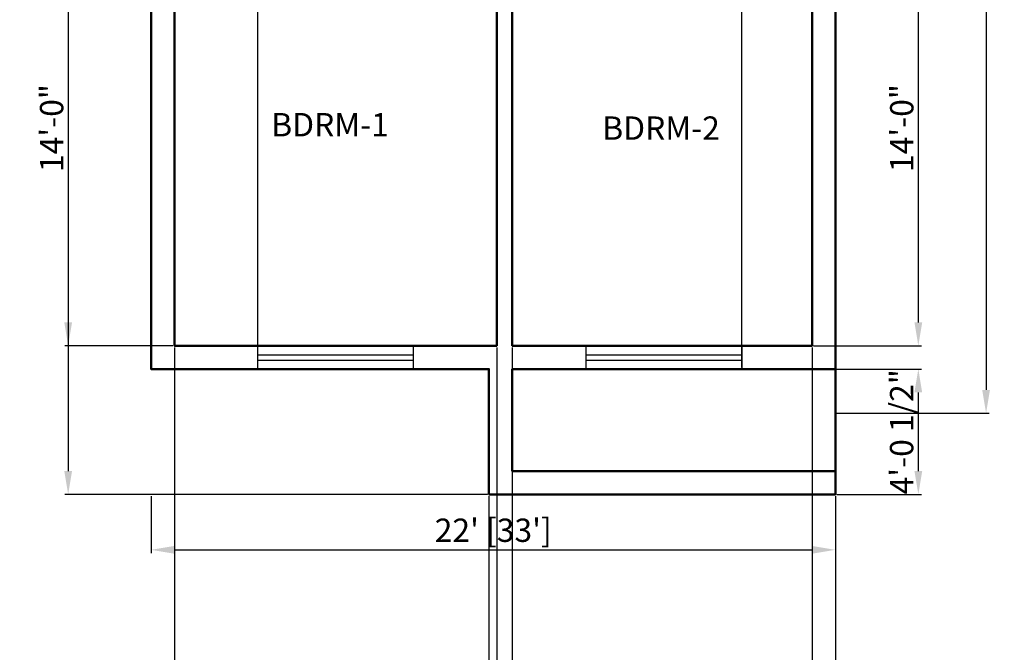
# Model space of a CAD drawing. Units: inches. Extents: x 2429 to 3343, y 1496 to 2530.
# Tile 5 of 7: x 2954 to 3334, y 1910 to 2154. Entities that reach past the tile are written whole.
import ezdxf

# ---------------------------------------------------------------- set-up
doc = ezdxf.new("R2010")
doc.units = ezdxf.units.IN
for name, color, linetype, lineweight in [('A-ANNO-DIMS', 2, 'Continuous', 18), ('A-AREA-IDEN', 3, 'Continuous', 18), ('A-GLAZ', 4, 'Continuous', 25), ('A-WALL', 7, 'Continuous', 50)]:
    doc.layers.add(name, color=color, linetype=linetype, lineweight=lineweight)
doc.styles.get("Standard").update_dxf_attribs({"font": 'arial.ttf'})
doc.dimstyles.new('ISO-25', dxfattribs={"dimtxt": 9, "dimasz": 9, "dimexe": 1.25, "dimexo": 0.625, "dimtad": 1, "dimdec": 1, "dimlunit": 3, "dimtxsty": 'Standard', "dimcen": 9, "dimadec": 0, "dimazin": 0, "dimtfac": 1, "dimtdec": 1, "dimtmove": 0, "dimatfit": 3, "dimfxl": 1, "dimarcsym": 0})

# ---------------------------------------------------------------- blocks, each defined once
blk = doc.blocks.new('*D8')
at = {"layer": 'A-ANNO-DIMS', "color": 0, "lineweight": -2, "transparency": 16777216}
for p, q in [((3005.05, 1969.85), (3005.05, 1947.84)), ((3269.05, 1969.85), (3269.05, 1947.84)), ((3014.05, 1949.09), (3260.05, 1949.09))]:
    blk.add_line(p, q, dxfattribs=at)
at = {"layer": 'A-ANNO-DIMS', "color": 0, "transparency": 16777216}
for points in [[(3014.05, 1950.59), (3014.05, 1947.59), (3005.05, 1949.09)], [(3260.05, 1950.59), (3260.05, 1947.59), (3269.05, 1949.09)]]:
    blk.add_solid(points, dxfattribs=at)
at = {"layer": 'Defpoints', "color": 0, "transparency": 16777216}
for p in [(3005.05, 1970.47), (3269.05, 1970.47), (3269.05, 1949.09)]:
    blk.add_point(p, dxfattribs=at)
at = {"layer": 'A-ANNO-DIMS', "color": 0, "transparency": 16777216, "insert": (3137.05, 1955.48), "char_height": 9, "attachment_point": 5}
blk.add_mtext("22' [33']", dxfattribs=at)
blk = doc.blocks.new('*D10')
at = {"layer": 'A-ANNO-DIMS', "color": 0, "lineweight": -2, "transparency": 16777216}
for p, q in [((3270.09, 2478.79), (3328.44, 2478.79)), ((3327.19, 2469.79), (3327.19, 2010.79)), ((3269.67, 2001.79), (3328.44, 2001.79))]:
    blk.add_line(p, q, dxfattribs=at)
at = {"layer": 'A-ANNO-DIMS', "color": 0, "transparency": 16777216}
for points in [[(3325.69, 2469.79), (3328.69, 2469.79), (3327.19, 2478.79)], [(3325.69, 2010.79), (3328.69, 2010.79), (3327.19, 2001.79)]]:
    blk.add_solid(points, dxfattribs=at)
at = {"layer": 'Defpoints', "color": 0, "transparency": 16777216}
for p in [(3269.47, 2478.79), (3269.05, 2001.79), (3327.19, 2001.79)]:
    blk.add_point(p, dxfattribs=at)
at = {"layer": 'A-ANNO-DIMS', "color": 0, "transparency": 16777216, "insert": (3320.8, 2240.29), "char_height": 9, "attachment_point": 5, "rotation": 90}
blk.add_mtext('39\'-9" [59\'-7.5"]', dxfattribs=at)
blk = doc.blocks.new('WIN-PLAN-1500')
for p, q in [((3.5, 60), (3.5, 0)), ((5.5, 60), (5.5, 0))]:
    blk.add_line(p, q)
blk.add_lwpolyline([(9, 60), (9, 0), (0, 0), (0, 60)], close=True)
blk = doc.blocks.new('*D56')
at = {"layer": 'A-ANNO-DIMS', "color": 0, "lineweight": -2, "transparency": 16777216}
for p, q in [((3004.42, 2478.79), (2971.8, 2478.79)), ((2973.05, 2469.79), (2973.05, 1979.47)), ((3134.79, 1970.47), (2971.8, 1970.47))]:
    blk.add_line(p, q, dxfattribs=at)
at = {"layer": 'A-ANNO-DIMS', "color": 0, "transparency": 16777216}
for points in [[(2971.55, 2469.79), (2974.55, 2469.79), (2973.05, 2478.79)], [(2971.55, 1979.47), (2974.55, 1979.47), (2973.05, 1970.47)]]:
    blk.add_solid(points, dxfattribs=at)
at = {"layer": 'Defpoints', "color": 0, "transparency": 16777216}
for p in [(3005.05, 2478.79), (2973.05, 1970.47), (3135.41, 1970.47)]:
    blk.add_point(p, dxfattribs=at)
at = {"layer": 'A-ANNO-DIMS', "color": 0, "transparency": 16777216, "insert": (2967.77, 2224.63), "char_height": 9, "attachment_point": 5, "rotation": 90}
blk.add_mtext('42\'-4 1/2"', dxfattribs=at)
blk = doc.blocks.new('*D65')
at = {"layer": 'A-ANNO-DIMS', "color": 0, "lineweight": -2, "transparency": 16777216}
for p, q in [((3014.05, 2027.16), (3014.05, 1860.42)), ((3138.41, 2027.16), (3138.41, 1860.42)), ((3023.05, 1861.67), (3129.41, 1861.67))]:
    blk.add_line(p, q, dxfattribs=at)
at = {"layer": 'A-ANNO-DIMS', "color": 0, "transparency": 16777216}
for points in [[(3023.05, 1863.17), (3023.05, 1860.17), (3014.05, 1861.67)], [(3129.41, 1863.17), (3129.41, 1860.17), (3138.41, 1861.67)]]:
    blk.add_solid(points, dxfattribs=at)
at = {"layer": 'Defpoints', "color": 0, "transparency": 16777216}
for p in [(3014.05, 2027.79), (3138.41, 2027.79), (3138.41, 1861.67)]:
    blk.add_point(p, dxfattribs=at)
at = {"layer": 'A-ANNO-DIMS', "color": 0, "transparency": 16777216, "insert": (3076.23, 1866.95), "char_height": 9, "attachment_point": 5}
blk.add_mtext('10\'-4 1/2"', dxfattribs=at)
blk = doc.blocks.new('*D66')
at = {"layer": 'A-ANNO-DIMS', "color": 0, "lineweight": -2, "transparency": 16777216}
for p, q in [((3013.42, 2195.79), (2971.8, 2195.79)), ((2973.05, 2186.79), (2973.05, 2036.79)), ((3013.42, 2027.79), (2971.8, 2027.79))]:
    blk.add_line(p, q, dxfattribs=at)
at = {"layer": 'A-ANNO-DIMS', "color": 0, "transparency": 16777216}
for points in [[(2971.55, 2186.79), (2974.55, 2186.79), (2973.05, 2195.79)], [(2971.55, 2036.79), (2974.55, 2036.79), (2973.05, 2027.79)]]:
    blk.add_solid(points, dxfattribs=at)
at = {"layer": 'Defpoints', "color": 0, "transparency": 16777216}
for p in [(3014.05, 2195.79), (2973.05, 2027.79), (3014.05, 2027.79)]:
    blk.add_point(p, dxfattribs=at)
at = {"layer": 'A-ANNO-DIMS', "color": 0, "transparency": 16777216, "insert": (2967.83, 2111.79), "char_height": 9, "attachment_point": 5, "rotation": 90}
blk.add_mtext('14\'-0"', dxfattribs=at)
blk = doc.blocks.new('*D67')
at = {"layer": 'A-ANNO-DIMS', "color": 0, "lineweight": -2, "transparency": 16777216}
for p, q in [((3144.41, 2027.16), (3144.41, 1860.42)), ((3260.05, 2027.16), (3260.05, 1860.42)), ((3153.41, 1861.67), (3251.05, 1861.67))]:
    blk.add_line(p, q, dxfattribs=at)
at = {"layer": 'A-ANNO-DIMS', "color": 0, "transparency": 16777216}
for points in [[(3153.41, 1863.17), (3153.41, 1860.17), (3144.41, 1861.67)], [(3251.05, 1863.17), (3251.05, 1860.17), (3260.05, 1861.67)]]:
    blk.add_solid(points, dxfattribs=at)
at = {"layer": 'Defpoints', "color": 0, "transparency": 16777216}
for p in [(3144.41, 2027.79), (3260.05, 2027.79), (3260.05, 1861.67)]:
    blk.add_point(p, dxfattribs=at)
at = {"layer": 'A-ANNO-DIMS', "color": 0, "transparency": 16777216, "insert": (3202.23, 1866.95), "char_height": 9, "attachment_point": 5}
blk.add_mtext('9\'-7 1/2"', dxfattribs=at)
blk = doc.blocks.new('*D68')
at = {"layer": 'A-ANNO-DIMS', "color": 0, "lineweight": -2, "transparency": 16777216}
for p, q in [((3260.67, 2195.79), (3302.3, 2195.79)), ((3301.05, 2186.79), (3301.05, 2036.79)), ((3260.67, 2027.79), (3302.3, 2027.79))]:
    blk.add_line(p, q, dxfattribs=at)
at = {"layer": 'A-ANNO-DIMS', "color": 0, "transparency": 16777216}
for points in [[(3299.55, 2186.79), (3302.55, 2186.79), (3301.05, 2195.79)], [(3299.55, 2036.79), (3302.55, 2036.79), (3301.05, 2027.79)]]:
    blk.add_solid(points, dxfattribs=at)
at = {"layer": 'Defpoints', "color": 0, "transparency": 16777216}
for p in [(3260.05, 2195.79), (3260.05, 2027.79), (3301.05, 2027.79)]:
    blk.add_point(p, dxfattribs=at)
at = {"layer": 'A-ANNO-DIMS', "color": 0, "transparency": 16777216, "insert": (3295.83, 2111.79), "char_height": 9, "attachment_point": 5, "rotation": 90}
blk.add_mtext('14\'-0"', dxfattribs=at)
blk = doc.blocks.new('*D69')
at = {"layer": 'A-ANNO-DIMS', "color": 0, "lineweight": -2, "transparency": 16777216}
for p, q in [((3269.67, 2018.79), (3302.3, 2018.79)), ((3301.05, 2009.79), (3301.05, 1979.47)), ((3269.67, 1970.47), (3302.3, 1970.47))]:
    blk.add_line(p, q, dxfattribs=at)
at = {"layer": 'A-ANNO-DIMS', "color": 0, "transparency": 16777216}
for points in [[(3299.55, 2009.79), (3302.55, 2009.79), (3301.05, 2018.79)], [(3299.55, 1979.47), (3302.55, 1979.47), (3301.05, 1970.47)]]:
    blk.add_solid(points, dxfattribs=at)
at = {"layer": 'Defpoints', "color": 0, "transparency": 16777216}
for p in [(3269.05, 2018.79), (3269.05, 1970.47), (3301.05, 1970.47)]:
    blk.add_point(p, dxfattribs=at)
at = {"layer": 'A-ANNO-DIMS', "color": 0, "transparency": 16777216, "insert": (3295.77, 1994.63), "char_height": 9, "attachment_point": 5, "rotation": 90}
blk.add_mtext('4\'-0 1/2"', dxfattribs=at)
blk = doc.blocks.new('*D70')
at = {"layer": 'A-ANNO-DIMS', "color": 0, "lineweight": -2, "transparency": 16777216}
for p, q in [((3135.41, 1969.85), (3135.41, 1860.42)), ((3269.05, 1969.85), (3269.05, 1860.42)), ((3144.41, 1861.67), (3260.05, 1861.67))]:
    blk.add_line(p, q, dxfattribs=at)
at = {"layer": 'A-ANNO-DIMS', "color": 0, "transparency": 16777216}
for points in [[(3144.41, 1863.17), (3144.41, 1860.17), (3135.41, 1861.67)], [(3260.05, 1863.17), (3260.05, 1860.17), (3269.05, 1861.67)]]:
    blk.add_solid(points, dxfattribs=at)
at = {"layer": 'Defpoints', "color": 0, "transparency": 16777216}
for p in [(3135.41, 1970.47), (3269.05, 1970.47), (3269.05, 1861.67)]:
    blk.add_point(p, dxfattribs=at)
at = {"layer": 'A-ANNO-DIMS', "color": 0, "transparency": 16777216, "insert": (3202.23, 1866.95), "char_height": 9, "attachment_point": 5}
blk.add_mtext('11\'-1 1/2"', dxfattribs=at)
blk = doc.blocks.new('*D76')
at = {"layer": 'A-ANNO-DIMS', "color": 0, "lineweight": -2, "transparency": 16777216}
for p, q in [((3005.05, 2019.41), (3005.05, 2512.04)), ((3046.2, 2019.41), (3046.2, 2512.04)), ((3014.05, 2510.79), (3037.2, 2510.79))]:
    blk.add_line(p, q, dxfattribs=at)
at = {"layer": 'A-ANNO-DIMS', "color": 0, "transparency": 16777216}
for points in [[(3014.05, 2512.29), (3014.05, 2509.29), (3005.05, 2510.79)], [(3037.2, 2512.29), (3037.2, 2509.29), (3046.2, 2510.79)]]:
    blk.add_solid(points, dxfattribs=at)
at = {"layer": 'Defpoints', "color": 0, "transparency": 16777216}
for p in [(3046.2, 2510.79), (3005.05, 2018.79), (3046.2, 2018.79)]:
    blk.add_point(p, dxfattribs=at)
at = {"layer": 'A-ANNO-DIMS', "color": 0, "transparency": 16777216, "insert": (3025.62, 2516.02), "char_height": 9, "attachment_point": 5}
blk.add_mtext('3\'-5"', dxfattribs=at)
blk = doc.blocks.new('*D77')
at = {"layer": 'A-ANNO-DIMS', "color": 0, "lineweight": -2, "transparency": 16777216}
for p, q in [((3232.91, 2019.41), (3232.91, 2512.04)), ((3269.05, 2019.41), (3269.05, 2512.04)), ((3241.91, 2510.79), (3260.05, 2510.79))]:
    blk.add_line(p, q, dxfattribs=at)
at = {"layer": 'A-ANNO-DIMS', "color": 0, "transparency": 16777216}
for points in [[(3241.91, 2512.29), (3241.91, 2509.29), (3232.91, 2510.79)], [(3260.05, 2512.29), (3260.05, 2509.29), (3269.05, 2510.79)]]:
    blk.add_solid(points, dxfattribs=at)
at = {"layer": 'Defpoints', "color": 0, "transparency": 16777216}
for p in [(3269.05, 2510.79), (3232.91, 2018.79), (3269.05, 2018.79)]:
    blk.add_point(p, dxfattribs=at)
at = {"layer": 'A-ANNO-DIMS', "color": 0, "transparency": 16777216, "insert": (3250.98, 2516.02), "char_height": 9, "attachment_point": 5}
blk.add_mtext('3\'-0"', dxfattribs=at)

msp = doc.modelspace()

# ---------------------------------------------------------------- linework, layer by layer
at = {"layer": 'A-WALL'}
msp.add_lwpolyline([(3135.41055, 1970.47184), (3269.04839, 1970.47184), (3269.04839, 2001.78649), (3269.04839, 2325.78649), (3269.04839, 2478.7918), (3005.04839, 2478.7918), (3005.04839, 2325.78649), (3005.04839, 2319.78649), (3005.04839, 2199.78649), (3005.04839, 2018.78649), (3135.41055, 2018.78649)], close=True, dxfattribs=at)
for points in [[(3133.9665, 2195.78649), (3138.41055, 2195.78649), (3138.41055, 2027.78649), (3014.04839, 2027.78649), (3014.04839, 2195.78649), (3099.7165, 2195.78649)], [(3185.96707, 2195.78649), (3260.04839, 2195.78649), (3260.04839, 2027.78649), (3144.41055, 2027.78649), (3144.41055, 2195.78649), (3151.71707, 2195.78649)], [(3269.04839, 1979.47184), (3144.41055, 1979.47184), (3144.41055, 2018.78649), (3269.04839, 2018.78649)]]:
    msp.add_lwpolyline(points, dxfattribs=at)

# ---------------------------------------------------------------- block references
at = {"layer": 'A-GLAZ'}
for p, rotation in [((3106.19932, 2018.78691), 90.00000000000048), ((3232.90581, 2018.78691), 90.00000000000115)]:
    msp.add_blockref('WIN-PLAN-1500', p, dxfattribs=dict(at, rotation=rotation))

# ---------------------------------------------------------------- texts
at = {"layer": 'A-AREA-IDEN', "char_height": 9, "attachment_point": 1}
for s, insert in [('{\\fCalibri|b0|i0|c0|p34;BDRM-1}', (3051.4096, 2117.58927)), ('{\\fCalibri|b0|i0|c0|p34;BDRM-2}', (3179.11755, 2116.27636))]:
    msp.add_mtext_dynamic_manual_height_columns(s, width=51.2251285, gutter_width=12.5, heights=[0], dxfattribs=dict(at, insert=insert))

# ---------------------------------------------------------------- dimensions: what is measured, and where the dimension line sits
at = {"layer": 'A-ANNO-DIMS'}
for base, p1, p2, override, picture, middle in [((3046.19896, 2510.7918), (3005.04839, 2018.78649), (3046.19896, 2018.78649), {"dimdec": 1, "dimlfac": 1, "dimrnd": 0, "dimzin": 1, "dimdsep": 46, "dimlunit": 4, "dimfrac": 2}, '*D76', (3025.62368, 2516.01503)), ((3269.04839, 2510.7918), (3232.90545, 2018.78649), (3269.04839, 2018.78649), {"dimdec": 1, "dimlfac": 1, "dimrnd": 0, "dimzin": 1, "dimdsep": 46, "dimlunit": 4, "dimfrac": 2}, '*D77', (3250.97692, 2516.01503)), ((3138.41055, 1861.66916), (3014.04839, 2027.78649), (3138.41055, 2027.78649), {"dimdec": 1, "dimlfac": 1, "dimrnd": 0, "dimzin": 1, "dimdsep": 46, "dimlunit": 4, "dimfrac": 2}, '*D65', (3076.22947, 1866.94764)), ((3260.04839, 1861.66916), (3144.41055, 2027.78649), (3260.04839, 2027.78649), {"dimdec": 1, "dimlfac": 1, "dimrnd": 0, "dimzin": 1, "dimdsep": 46, "dimlunit": 4, "dimfrac": 2}, '*D67', (3202.22947, 1866.94764)), ((3269.04839, 1949.08895), (3005.04839, 1970.47184), (3269.04839, 1970.47184), {"dimclrd": 0, "dimclre": 0, "dimclrt": 0}, '*D8', (3137.04839, 1955.48169)), ((3269.04839, 1861.66916), (3135.41055, 1970.47184), (3269.04839, 1970.47184), {"dimdec": 1, "dimlfac": 1, "dimrnd": 0, "dimzin": 1, "dimdsep": 46, "dimlunit": 4, "dimfrac": 2}, '*D70', (3202.22947, 1866.94764))]:
    dim = msp.add_linear_dim(base=base, p1=p1, p2=p2, dimstyle='ISO-25', override=override, dxfattribs=at)
    dim.commit()
    dim.dimension.update_dxf_attribs({"geometry": picture, "text_midpoint": middle})
for base, p1, p2, override, picture, middle in [((2973.04839, 1970.47184), (3005.04839, 2478.7918), (3135.41055, 1970.47184), {"dimdec": 1, "dimlfac": 1, "dimrnd": 0, "dimzin": 1, "dimdsep": 46, "dimlunit": 4, "dimfrac": 2}, '*D56', (2967.76991, 2224.63182)), ((3327.19291, 2001.78649), (3269.46607, 2478.7918), (3269.04839, 2001.78649), {"dimclrd": 0, "dimclre": 0, "dimclrt": 0}, '*D10', (3320.80018, 2240.28915)), ((2973.04839, 2027.78649), (3014.04839, 2195.78649), (3014.04839, 2027.78649), {"dimdec": 1, "dimlfac": 1, "dimrnd": 0, "dimzin": 1, "dimdsep": 46, "dimlunit": 4, "dimfrac": 2}, '*D66', (2967.82824, 2111.78649)), ((3301.04839, 2027.78649), (3260.04839, 2195.78649), (3260.04839, 2027.78649), {"dimdec": 1, "dimlfac": 1, "dimrnd": 0, "dimzin": 1, "dimdsep": 46, "dimlunit": 4, "dimfrac": 2}, '*D68', (3295.82824, 2111.78649)), ((3301.04839, 1970.47184), (3269.04839, 2018.78649), (3269.04839, 1970.47184), {"dimdec": 1, "dimlfac": 1, "dimrnd": 0, "dimzin": 1, "dimdsep": 46, "dimlunit": 4, "dimfrac": 2}, '*D69', (3295.76991, 1994.62916))]:
    dim = msp.add_linear_dim(base=base, p1=p1, p2=p2, angle=90, dimstyle='ISO-25', override=override, dxfattribs=at)
    dim.commit()
    dim.dimension.update_dxf_attribs({"geometry": picture, "text_midpoint": middle})

doc.saveas('drawing.dxf')
